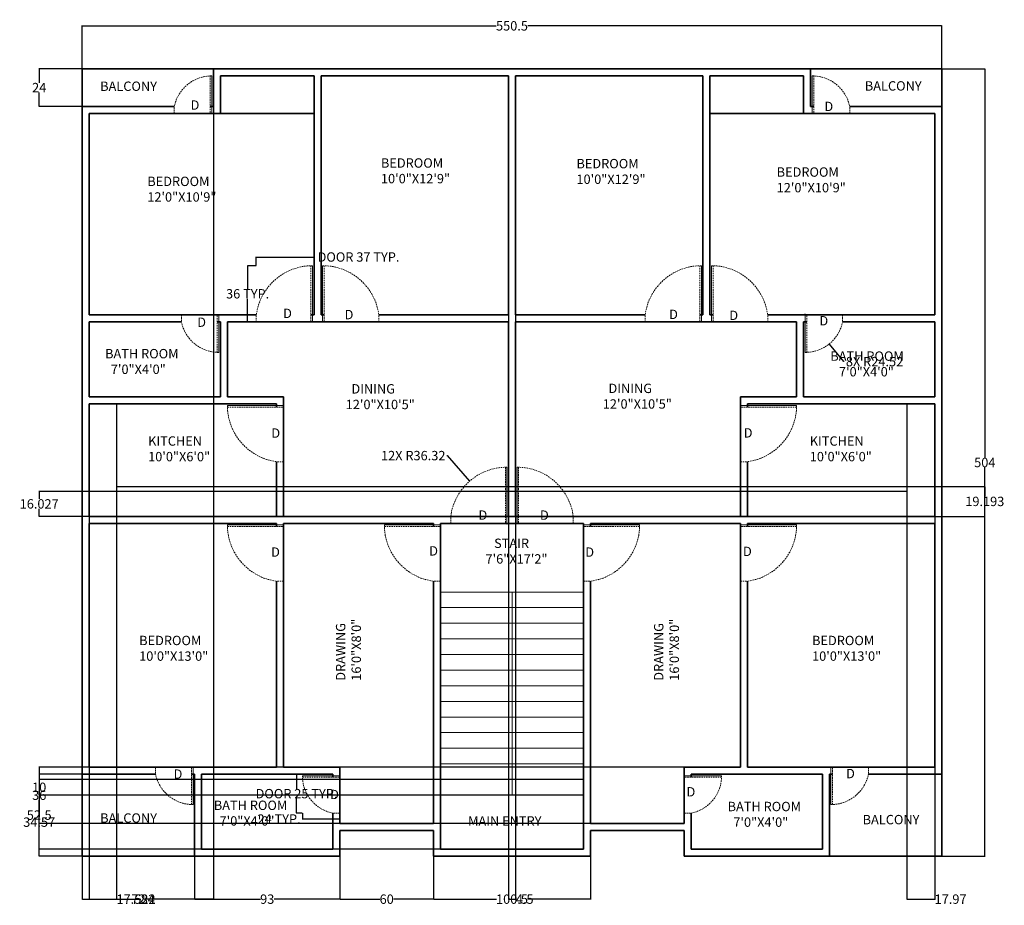
# Model space of a CAD drawing. Units: inches. Extents: x 4870 to 5501, y 14934 to 15501.
import ezdxf

# ---------------------------------------------------------------- set-up
doc = ezdxf.new("R2010")
doc.units = ezdxf.units.IN
doc.header["$MEASUREMENT"] = 0
doc.linetypes.add('DASHEDX2', pattern=[1.5, 1, -0.5])
for name, color, linetype, lineweight in [('A-ANNO-DIMS', 2, 'Continuous', 18), ('A-ANNO-TEXT', 7, 'Continuous', 18), ('A-AREA-IDEN', 7, 'Continuous', 18), ('A-DOOR', 4, 'DASHEDX2', 18), ('A-FLOR-FIXT', 8, 'Continuous', 18), ('A-FLOR-STRS', 7, 'Continuous', 18), ('A-WALL', 7, 'Continuous', 35)]:
    doc.layers.add(name, color=color, linetype=linetype, lineweight=lineweight)
doc.styles.get("Standard").update_dxf_attribs({"font": 'arial.ttf'})
doc.dimstyles.get("Standard").update_dxf_attribs({"dimtxt": 6, "dimasz": 0.18, "dimexe": 0.18, "dimexo": 0.0625, "dimgap": 0.09, "dimtad": 0, "dimtih": 1, "dimtoh": 1, "dimdec": 1, "dimzin": 0, "dimdsep": 46, "dimlunit": 3, "dimtxsty": 'Standard', "dimcen": 0.09, "dimadec": 0, "dimazin": 0, "dimtfac": 1, "dimtdec": 1, "dimtofl": 0, "dimtmove": 0, "dimatfit": 3, "dimfxl": 1, "dimtolj": 1, "dimtzin": 0, "dimarcsym": 0})

# ---------------------------------------------------------------- blocks, each defined once
blk = doc.blocks.new('DOOR-SWING-24IN')
for p, q in [((-1, 24), (-1, 0)), ((0, 0), (0, 24)), ((0, 24), (0, 0)), ((-24, 0), (-24, 4.5)), ((0, 0), (-24, 0)), ((1, 0), (0, 0))]:
    blk.add_line(p, q)
blk.add_arc((0, -0.52), 24.52, 90, 168.18772)
blk = doc.blocks.new('DOOR-SWING-36IN')
for p, q in [((-1, 36), (-1, 0)), ((0, 0), (0, 36)), ((0, 36), (0, 0)), ((-36, 0), (-36, 4.5)), ((0, 0), (-36, 0)), ((1, 0), (0, 0))]:
    blk.add_line(p, q)
blk.add_arc((0, -0.32), 36.32, 90, 172.37185)
blk = doc.blocks.new('*D3')
at = {"layer": 'A-ANNO-DIMS', "color": 0, "lineweight": -2, "transparency": 16777216}
for p, q in [((5021.91, 15343.26), (5021.91, 15348.93)), ((5022.09, 15348.75), (5058.73, 15348.75)), ((5058.91, 15343.26), (5058.91, 15348.93)), ((5058.91, 15348.75), (5059.09, 15348.75))]:
    blk.add_line(p, q, dxfattribs=at)
at = {"layer": 'A-ANNO-DIMS', "color": 0, "transparency": 16777216}
for points in [[(5022.09, 15348.78), (5022.09, 15348.72), (5021.91, 15348.75)], [(5058.73, 15348.78), (5058.73, 15348.72), (5058.91, 15348.75)]]:
    blk.add_solid(points, dxfattribs=at)
at = {"layer": 'Defpoints', "color": 0, "transparency": 16777216}
for p in [(5058.91, 15348.75), (5021.91, 15343.2), (5058.91, 15343.2)]:
    blk.add_point(p, dxfattribs=at)
at = {"layer": 'A-ANNO-DIMS', "color": 0, "transparency": 16777216, "insert": (5087.37, 15348.75), "char_height": 6, "attachment_point": 5}
blk.add_mtext('\\A1;DOOR 37 TYP.', dxfattribs=at)
blk = doc.blocks.new('*D4')
at = {"layer": 'A-ANNO-DIMS', "color": 0, "lineweight": -2, "transparency": 16777216}
for p, q in [((5021.85, 15343.2), (5016.18, 15343.2)), ((5016.36, 15343.02), (5016.36, 15328.35)), ((5016.36, 15307.38), (5016.36, 15322.04)), ((5021.85, 15307.2), (5016.18, 15307.2))]:
    blk.add_line(p, q, dxfattribs=at)
at = {"layer": 'A-ANNO-DIMS', "color": 0, "transparency": 16777216}
for points in [[(5016.33, 15343.02), (5016.39, 15343.02), (5016.36, 15343.2)], [(5016.33, 15307.38), (5016.39, 15307.38), (5016.36, 15307.2)]]:
    blk.add_solid(points, dxfattribs=at)
at = {"layer": 'Defpoints', "color": 0, "transparency": 16777216}
for p in [(5016.36, 15343.2), (5021.91, 15343.2), (5021.91, 15307.2)]:
    blk.add_point(p, dxfattribs=at)
at = {"layer": 'A-ANNO-DIMS', "color": 0, "transparency": 16777216, "insert": (5016.36, 15325.2), "char_height": 6, "attachment_point": 5}
blk.add_mtext('\\A1;36 TYP.', dxfattribs=at)
blk = doc.blocks.new('*D5')
at = {"layer": 'A-ANNO-DIMS', "color": 0, "lineweight": -2, "transparency": 16777216}
for p, q in [((5051.35, 15017.7), (5047.48, 15017.7)), ((5047.66, 15017.52), (5047.66, 15008.39)), ((5047.66, 14992.88), (5047.66, 15002)), ((5051.35, 14992.7), (5047.48, 14992.7))]:
    blk.add_line(p, q, dxfattribs=at)
at = {"layer": 'A-ANNO-DIMS', "color": 0, "transparency": 16777216}
for points in [[(5047.63, 15017.52), (5047.69, 15017.52), (5047.66, 15017.7)], [(5047.63, 14992.88), (5047.69, 14992.88), (5047.66, 14992.7)]]:
    blk.add_solid(points, dxfattribs=at)
at = {"layer": 'Defpoints', "color": 0, "transparency": 16777216}
for p in [(5047.66, 15017.7), (5051.41, 15017.7), (5051.41, 14992.7)]:
    blk.add_point(p, dxfattribs=at)
at = {"layer": 'A-ANNO-DIMS', "color": 0, "transparency": 16777216, "insert": (5047.66, 15005.2), "char_height": 6, "attachment_point": 5}
blk.add_mtext('\\A1;DOOR 25 TYP.', dxfattribs=at)
blk = doc.blocks.new('*D6')
at = {"layer": 'A-ANNO-DIMS', "color": 0, "lineweight": -2, "transparency": 16777216}
for p, q in [((5051.41, 14988.95), (5051.23, 14988.95)), ((5051.41, 14992.64), (5051.41, 14988.77)), ((5075.23, 14988.95), (5051.59, 14988.95)), ((5075.41, 14992.64), (5075.41, 14988.77))]:
    blk.add_line(p, q, dxfattribs=at)
at = {"layer": 'A-ANNO-DIMS', "color": 0, "transparency": 16777216}
for points in [[(5051.59, 14988.98), (5051.59, 14988.92), (5051.41, 14988.95)], [(5075.23, 14988.98), (5075.23, 14988.92), (5075.41, 14988.95)]]:
    blk.add_solid(points, dxfattribs=at)
at = {"layer": 'Defpoints', "color": 0, "transparency": 16777216}
for p in [(5051.41, 14992.7), (5051.41, 14988.95), (5075.41, 14992.7)]:
    blk.add_point(p, dxfattribs=at)
at = {"layer": 'A-ANNO-DIMS', "color": 0, "transparency": 16777216, "insert": (5036.49, 14988.95), "char_height": 6, "attachment_point": 5}
blk.add_mtext('\\A1;24 TYP.', dxfattribs=at)
blk = doc.blocks.new('*D7')
at = {"layer": 'A-ANNO-DIMS', "color": 0, "lineweight": -2, "transparency": 16777216}
for p, q in [((4910.41, 15469.26), (4910.41, 15496.91)), ((4910.59, 15496.73), (5175.43, 15496.73)), ((5460.73, 15496.73), (5195.9, 15496.73)), ((5460.91, 15469.26), (5460.91, 15496.91))]:
    blk.add_line(p, q, dxfattribs=at)
at = {"layer": 'A-ANNO-DIMS', "color": 0, "transparency": 16777216}
for points in [[(4910.59, 15496.76), (4910.59, 15496.7), (4910.41, 15496.73)], [(5460.73, 15496.76), (5460.73, 15496.7), (5460.91, 15496.73)]]:
    blk.add_solid(points, dxfattribs=at)
at = {"layer": 'Defpoints', "color": 0, "transparency": 16777216}
for p in [(5460.91, 15496.73), (4910.41, 15469.2), (5460.91, 15469.2)]:
    blk.add_point(p, dxfattribs=at)
at = {"layer": 'A-ANNO-DIMS', "color": 0, "transparency": 16777216, "insert": (5185.66, 15496.73), "char_height": 6, "attachment_point": 5}
blk.add_mtext('\\A1;550.5', dxfattribs=at)
blk = doc.blocks.new('*D8')
at = {"layer": 'A-ANNO-DIMS', "color": 0, "lineweight": -2, "transparency": 16777216}
for p, q in [((5460.97, 15469.2), (5488.62, 15469.2)), ((5488.44, 15469.02), (5488.44, 15220.35)), ((5488.44, 14965.38), (5488.44, 15214.04)), ((5460.97, 14965.2), (5488.62, 14965.2))]:
    blk.add_line(p, q, dxfattribs=at)
at = {"layer": 'A-ANNO-DIMS', "color": 0, "transparency": 16777216}
for points in [[(5488.41, 15469.02), (5488.47, 15469.02), (5488.44, 15469.2)], [(5488.41, 14965.38), (5488.47, 14965.38), (5488.44, 14965.2)]]:
    blk.add_solid(points, dxfattribs=at)
at = {"layer": 'Defpoints', "color": 0, "transparency": 16777216}
for p in [(5460.91, 15469.2), (5488.44, 15469.2), (5460.91, 14965.2)]:
    blk.add_point(p, dxfattribs=at)
at = {"layer": 'A-ANNO-DIMS', "color": 0, "transparency": 16777216, "insert": (5488.44, 15217.2), "char_height": 6, "attachment_point": 5}
blk.add_mtext('\\A1;504', dxfattribs=at)
blk = doc.blocks.new('*D9')
at = {"layer": 'A-ANNO-DIMS', "color": 0, "lineweight": -2, "transparency": 16777216}
for p, q in [((4910.41, 15469.14), (4910.41, 14937.49)), ((4994.41, 15469.14), (4994.41, 14937.49)), ((4910.59, 14937.67), (4948.03, 14937.67)), ((4994.23, 14937.67), (4956.79, 14937.67))]:
    blk.add_line(p, q, dxfattribs=at)
at = {"layer": 'A-ANNO-DIMS', "color": 0, "transparency": 16777216}
for points in [[(4910.59, 14937.7), (4910.59, 14937.64), (4910.41, 14937.67)], [(4994.23, 14937.7), (4994.23, 14937.64), (4994.41, 14937.67)]]:
    blk.add_solid(points, dxfattribs=at)
at = {"layer": 'Defpoints', "color": 0, "transparency": 16777216}
for p in [(4910.41, 15469.2), (4994.41, 15469.2), (4994.41, 14937.67)]:
    blk.add_point(p, dxfattribs=at)
at = {"layer": 'A-ANNO-DIMS', "color": 0, "transparency": 16777216, "insert": (4952.41, 14937.67), "char_height": 6, "attachment_point": 5}
blk.add_mtext('\\A1;84', dxfattribs=at)
blk = doc.blocks.new('*D10')
at = {"layer": 'A-ANNO-DIMS', "color": 0, "lineweight": -2, "transparency": 16777216}
for p, q in [((4910.35, 15469.2), (4882.7, 15469.2)), ((4882.88, 15469.02), (4882.88, 15460.3)), ((4882.88, 15445.38), (4882.88, 15454.1)), ((4910.35, 15445.2), (4882.7, 15445.2))]:
    blk.add_line(p, q, dxfattribs=at)
at = {"layer": 'A-ANNO-DIMS', "color": 0, "transparency": 16777216}
for points in [[(4882.85, 15469.02), (4882.91, 15469.02), (4882.88, 15469.2)], [(4882.85, 15445.38), (4882.91, 15445.38), (4882.88, 15445.2)]]:
    blk.add_solid(points, dxfattribs=at)
at = {"layer": 'Defpoints', "color": 0, "transparency": 16777216}
for p in [(4882.88, 15469.2), (4910.41, 15469.2), (4910.41, 15445.2)]:
    blk.add_point(p, dxfattribs=at)
at = {"layer": 'A-ANNO-DIMS', "color": 0, "transparency": 16777216, "insert": (4882.88, 15457.2), "char_height": 6, "attachment_point": 5}
blk.add_mtext('\\A1;24', dxfattribs=at)
blk = doc.blocks.new('*D11')
at = {"layer": 'A-ANNO-DIMS', "color": 0, "lineweight": -2, "transparency": 16777216}
for p, q in [((4910.41, 14965.14), (4910.41, 14937.49)), ((4982.41, 14965.14), (4982.41, 14937.49)), ((4910.59, 14937.67), (4942.08, 14937.67)), ((4982.23, 14937.67), (4950.74, 14937.67))]:
    blk.add_line(p, q, dxfattribs=at)
at = {"layer": 'A-ANNO-DIMS', "color": 0, "transparency": 16777216}
for points in [[(4910.59, 14937.7), (4910.59, 14937.64), (4910.41, 14937.67)], [(4982.23, 14937.7), (4982.23, 14937.64), (4982.41, 14937.67)]]:
    blk.add_solid(points, dxfattribs=at)
at = {"layer": 'Defpoints', "color": 0, "transparency": 16777216}
for p in [(4910.41, 14965.2), (4982.41, 14965.2), (4982.41, 14937.67)]:
    blk.add_point(p, dxfattribs=at)
at = {"layer": 'A-ANNO-DIMS', "color": 0, "transparency": 16777216, "insert": (4946.41, 14937.67), "char_height": 6, "attachment_point": 5}
blk.add_mtext('\\A1;72', dxfattribs=at)
blk = doc.blocks.new('*D12')
at = {"layer": 'A-ANNO-DIMS', "color": 0, "lineweight": -2, "transparency": 16777216}
for p, q in [((4910.35, 15017.7), (4882.7, 15017.7)), ((4882.88, 15017.52), (4882.88, 14994.6)), ((4882.88, 14965.38), (4882.88, 14988.29)), ((4910.35, 14965.2), (4882.7, 14965.2))]:
    blk.add_line(p, q, dxfattribs=at)
at = {"layer": 'A-ANNO-DIMS', "color": 0, "transparency": 16777216}
for points in [[(4882.85, 15017.52), (4882.91, 15017.52), (4882.88, 15017.7)], [(4882.85, 14965.38), (4882.91, 14965.38), (4882.88, 14965.2)]]:
    blk.add_solid(points, dxfattribs=at)
at = {"layer": 'Defpoints', "color": 0, "transparency": 16777216}
for p in [(4882.88, 15017.7), (4910.41, 15017.7), (4910.41, 14965.2)]:
    blk.add_point(p, dxfattribs=at)
at = {"layer": 'A-ANNO-DIMS', "color": 0, "transparency": 16777216, "insert": (4882.88, 14991.45), "char_height": 6, "attachment_point": 5}
blk.add_mtext('\\A1;52.5', dxfattribs=at)
blk = doc.blocks.new('*D13')
at = {"layer": 'A-ANNO-DIMS', "color": 0, "lineweight": -2, "transparency": 16777216}
for p, q in [((4982.41, 14965.14), (4982.41, 14937.49)), ((5075.41, 14965.14), (5075.41, 14937.49)), ((4982.59, 14937.67), (5024.52, 14937.67)), ((5075.23, 14937.67), (5033.3, 14937.67))]:
    blk.add_line(p, q, dxfattribs=at)
at = {"layer": 'A-ANNO-DIMS', "color": 0, "transparency": 16777216}
for points in [[(4982.59, 14937.7), (4982.59, 14937.64), (4982.41, 14937.67)], [(5075.23, 14937.7), (5075.23, 14937.64), (5075.41, 14937.67)]]:
    blk.add_solid(points, dxfattribs=at)
at = {"layer": 'Defpoints', "color": 0, "transparency": 16777216}
for p in [(4982.41, 14965.2), (5075.41, 14965.2), (5075.41, 14937.67)]:
    blk.add_point(p, dxfattribs=at)
at = {"layer": 'A-ANNO-DIMS', "color": 0, "transparency": 16777216, "insert": (5028.91, 14937.67), "char_height": 6, "attachment_point": 5}
blk.add_mtext('\\A1;93', dxfattribs=at)
blk = doc.blocks.new('*D14')
at = {"layer": 'A-ANNO-DIMS', "color": 0, "lineweight": -2, "transparency": 16777216}
for p, q in [((5075.41, 14965.14), (5075.41, 14937.49)), ((5135.41, 14965.14), (5135.41, 14937.49)), ((5075.59, 14937.67), (5101.02, 14937.67)), ((5135.23, 14937.67), (5109.81, 14937.67))]:
    blk.add_line(p, q, dxfattribs=at)
at = {"layer": 'A-ANNO-DIMS', "color": 0, "transparency": 16777216}
for points in [[(5075.59, 14937.7), (5075.59, 14937.64), (5075.41, 14937.67)], [(5135.23, 14937.7), (5135.23, 14937.64), (5135.41, 14937.67)]]:
    blk.add_solid(points, dxfattribs=at)
at = {"layer": 'Defpoints', "color": 0, "transparency": 16777216}
for p in [(5075.41, 14965.2), (5135.41, 14965.2), (5135.41, 14937.67)]:
    blk.add_point(p, dxfattribs=at)
at = {"layer": 'A-ANNO-DIMS', "color": 0, "transparency": 16777216, "insert": (5105.41, 14937.67), "char_height": 6, "attachment_point": 5}
blk.add_mtext('\\A1;60', dxfattribs=at)
blk = doc.blocks.new('*D15')
at = {"layer": 'A-ANNO-DIMS', "color": 0, "lineweight": -2, "transparency": 16777216}
for p, q in [((5135.41, 14965.14), (5135.41, 14937.49)), ((5235.91, 14965.14), (5235.91, 14937.49)), ((5135.59, 14937.67), (5175.71, 14937.67)), ((5235.73, 14937.67), (5195.62, 14937.67))]:
    blk.add_line(p, q, dxfattribs=at)
at = {"layer": 'A-ANNO-DIMS', "color": 0, "transparency": 16777216}
for points in [[(5135.59, 14937.7), (5135.59, 14937.64), (5135.41, 14937.67)], [(5235.73, 14937.7), (5235.73, 14937.64), (5235.91, 14937.67)]]:
    blk.add_solid(points, dxfattribs=at)
at = {"layer": 'Defpoints', "color": 0, "transparency": 16777216}
for p in [(5135.41, 14965.2), (5235.91, 14965.2), (5235.91, 14937.67)]:
    blk.add_point(p, dxfattribs=at)
at = {"layer": 'A-ANNO-DIMS', "color": 0, "transparency": 16777216, "insert": (5185.66, 14937.67), "char_height": 6, "attachment_point": 5}
blk.add_mtext('\\A1;100.5', dxfattribs=at)
blk = doc.blocks.new('*D16')
at = {"layer": 'A-ANNO-DIMS', "color": 0, "lineweight": -2, "transparency": 16777216}
for p, q in [((5295.85, 15022.2), (4882.7, 15022.2)), ((4882.88, 15022.02), (4882.88, 15007.35)), ((4882.88, 14986.38), (4882.88, 15001.04)), ((5295.85, 14986.2), (4882.7, 14986.2))]:
    blk.add_line(p, q, dxfattribs=at)
at = {"layer": 'A-ANNO-DIMS', "color": 0, "transparency": 16777216}
for points in [[(4882.85, 15022.02), (4882.91, 15022.02), (4882.88, 15022.2)], [(4882.85, 14986.38), (4882.91, 14986.38), (4882.88, 14986.2)]]:
    blk.add_solid(points, dxfattribs=at)
at = {"layer": 'Defpoints', "color": 0, "transparency": 16777216}
for p in [(4882.88, 15022.2), (5295.91, 15022.2), (5295.91, 14986.2)]:
    blk.add_point(p, dxfattribs=at)
at = {"layer": 'A-ANNO-DIMS', "color": 0, "transparency": 16777216, "insert": (4882.88, 15004.2), "char_height": 6, "attachment_point": 5}
blk.add_mtext('\\A1;36', dxfattribs=at)
blk = doc.blocks.new('*D17')
at = {"layer": 'A-ANNO-DIMS', "color": 0, "lineweight": -2, "transparency": 16777216}
for p, q in [((5231.35, 15004.27), (4882.7, 15004.27)), ((4882.88, 15004.09), (4882.88, 14990.14)), ((4882.88, 14969.88), (4882.88, 14983.83)), ((5231.35, 14969.7), (4882.7, 14969.7))]:
    blk.add_line(p, q, dxfattribs=at)
at = {"layer": 'A-ANNO-DIMS', "color": 0, "transparency": 16777216}
for points in [[(4882.85, 15004.09), (4882.91, 15004.09), (4882.88, 15004.27)], [(4882.85, 14969.88), (4882.91, 14969.88), (4882.88, 14969.7)]]:
    blk.add_solid(points, dxfattribs=at)
at = {"layer": 'Defpoints', "color": 0, "transparency": 16777216}
for p in [(4882.88, 15004.27), (5231.41, 15004.27), (5231.41, 14969.7)]:
    blk.add_point(p, dxfattribs=at)
at = {"layer": 'A-ANNO-DIMS', "color": 0, "transparency": 16777216, "insert": (4882.88, 14986.98), "char_height": 6, "attachment_point": 5}
blk.add_mtext('\\A1;34.57', dxfattribs=at)
blk = doc.blocks.new('*D18')
at = {"layer": 'A-ANNO-DIMS', "color": 0, "lineweight": -2, "transparency": 16777216}
for p, q in [((5231.35, 15014.27), (4882.7, 15014.27)), ((4882.88, 15014.09), (4882.88, 15012.42)), ((5231.35, 15004.27), (4882.7, 15004.27)), ((4882.88, 15004.45), (4882.88, 15006.12))]:
    blk.add_line(p, q, dxfattribs=at)
at = {"layer": 'A-ANNO-DIMS', "color": 0, "transparency": 16777216}
for points in [[(4882.85, 15014.09), (4882.91, 15014.09), (4882.88, 15014.27)], [(4882.85, 15004.45), (4882.91, 15004.45), (4882.88, 15004.27)]]:
    blk.add_solid(points, dxfattribs=at)
at = {"layer": 'Defpoints', "color": 0, "transparency": 16777216}
for p in [(4882.88, 15014.27), (5231.41, 15014.27), (5231.41, 15004.27)]:
    blk.add_point(p, dxfattribs=at)
at = {"layer": 'A-ANNO-DIMS', "color": 0, "transparency": 16777216, "insert": (4882.88, 15009.27), "char_height": 6, "attachment_point": 5}
blk.add_mtext('\\A1;10', dxfattribs=at)
blk = doc.blocks.new('*D19')
at = {"layer": 'A-ANNO-DIMS', "color": 0, "lineweight": -2, "transparency": 16777216}
for p, q in [((5183.41, 15464.64), (5183.41, 14937.49)), ((5187.91, 15464.64), (5187.91, 14937.49)), ((5183.59, 14937.67), (5187.73, 14937.67)), ((5187.91, 14937.67), (5188.09, 14937.67))]:
    blk.add_line(p, q, dxfattribs=at)
at = {"layer": 'A-ANNO-DIMS', "color": 0, "transparency": 16777216}
for points in [[(5183.59, 14937.7), (5183.59, 14937.64), (5183.41, 14937.67)], [(5187.73, 14937.7), (5187.73, 14937.64), (5187.91, 14937.67)]]:
    blk.add_solid(points, dxfattribs=at)
at = {"layer": 'Defpoints', "color": 0, "transparency": 16777216}
for p in [(5183.41, 15464.7), (5187.91, 15464.7), (5187.91, 14937.67)]:
    blk.add_point(p, dxfattribs=at)
at = {"layer": 'A-ANNO-DIMS', "color": 0, "transparency": 16777216, "insert": (5193.79, 14937.67), "char_height": 6, "attachment_point": 5}
blk.add_mtext('\\A1;4.5', dxfattribs=at)
blk = doc.blocks.new('*D20')
at = {"layer": 'A-ANNO-DIMS', "color": 0, "lineweight": -2, "transparency": 16777216}
for p, q in [((4914.91, 15254.64), (4914.91, 14937.49)), ((4932.43, 15254.64), (4932.43, 14937.49)), ((4915.09, 14937.67), (4932.25, 14937.67)), ((4932.43, 14937.67), (4932.61, 14937.67))]:
    blk.add_line(p, q, dxfattribs=at)
at = {"layer": 'A-ANNO-DIMS', "color": 0, "transparency": 16777216}
for points in [[(4915.09, 14937.7), (4915.09, 14937.64), (4914.91, 14937.67)], [(4932.25, 14937.7), (4932.25, 14937.64), (4932.43, 14937.67)]]:
    blk.add_solid(points, dxfattribs=at)
at = {"layer": 'Defpoints', "color": 0, "transparency": 16777216}
for p in [(4914.91, 15254.7), (4932.43, 15254.7), (4932.43, 14937.67)]:
    blk.add_point(p, dxfattribs=at)
at = {"layer": 'A-ANNO-DIMS', "color": 0, "transparency": 16777216, "insert": (4944.85, 14937.67), "char_height": 6, "attachment_point": 5}
blk.add_mtext('\\A1;17.522', dxfattribs=at)
blk = doc.blocks.new('*D21')
at = {"layer": 'A-ANNO-DIMS', "color": 0, "lineweight": -2, "transparency": 16777216}
for p, q in [((4932.5, 15201.89), (5488.62, 15201.89)), ((5488.44, 15201.71), (5488.44, 15195.45)), ((5488.44, 15182.88), (5488.44, 15189.14)), ((4914.97, 15182.7), (5488.62, 15182.7))]:
    blk.add_line(p, q, dxfattribs=at)
at = {"layer": 'A-ANNO-DIMS', "color": 0, "transparency": 16777216}
for points in [[(5488.41, 15201.71), (5488.47, 15201.71), (5488.44, 15201.89)], [(5488.41, 15182.88), (5488.47, 15182.88), (5488.44, 15182.7)]]:
    blk.add_solid(points, dxfattribs=at)
at = {"layer": 'Defpoints', "color": 0, "transparency": 16777216}
for p in [(4932.43, 15201.89), (5488.44, 15201.89), (4914.91, 15182.7)]:
    blk.add_point(p, dxfattribs=at)
at = {"layer": 'A-ANNO-DIMS', "color": 0, "transparency": 16777216, "insert": (5488.44, 15192.29), "char_height": 6, "attachment_point": 5}
blk.add_mtext('\\A1;19.193', dxfattribs=at)
blk = doc.blocks.new('*D22')
at = {"layer": 'A-ANNO-DIMS', "color": 0, "lineweight": -2, "transparency": 16777216}
for p, q in [((5438.44, 15254.64), (5438.44, 14937.49)), ((5456.41, 15254.64), (5456.41, 14937.49)), ((5438.62, 14937.67), (5456.23, 14937.67)), ((5456.41, 14937.67), (5456.59, 14937.67))]:
    blk.add_line(p, q, dxfattribs=at)
at = {"layer": 'A-ANNO-DIMS', "color": 0, "transparency": 16777216}
for points in [[(5438.62, 14937.7), (5438.62, 14937.64), (5438.44, 14937.67)], [(5456.23, 14937.7), (5456.23, 14937.64), (5456.41, 14937.67)]]:
    blk.add_solid(points, dxfattribs=at)
at = {"layer": 'Defpoints', "color": 0, "transparency": 16777216}
for p in [(5438.44, 15254.7), (5456.41, 15254.7), (5456.41, 14937.67)]:
    blk.add_point(p, dxfattribs=at)
at = {"layer": 'A-ANNO-DIMS', "color": 0, "transparency": 16777216, "insert": (5466.52, 14937.67), "char_height": 6, "attachment_point": 5}
blk.add_mtext('\\A1;17.97', dxfattribs=at)
blk = doc.blocks.new('*D23')
at = {"layer": 'A-ANNO-DIMS', "color": 0, "lineweight": -2, "transparency": 16777216}
for p, q in [((5438.38, 15198.73), (4882.7, 15198.73)), ((4882.88, 15198.55), (4882.88, 15193.86)), ((4882.88, 15182.88), (4882.88, 15187.56)), ((5456.35, 15182.7), (4882.7, 15182.7))]:
    blk.add_line(p, q, dxfattribs=at)
at = {"layer": 'A-ANNO-DIMS', "color": 0, "transparency": 16777216}
for points in [[(4882.85, 15198.55), (4882.91, 15198.55), (4882.88, 15198.73)], [(4882.85, 15182.88), (4882.91, 15182.88), (4882.88, 15182.7)]]:
    blk.add_solid(points, dxfattribs=at)
at = {"layer": 'Defpoints', "color": 0, "transparency": 16777216}
for p in [(5438.44, 15198.73), (4882.88, 15182.7), (5456.41, 15182.7)]:
    blk.add_point(p, dxfattribs=at)
at = {"layer": 'A-ANNO-DIMS', "color": 0, "transparency": 16777216, "insert": (4882.88, 15190.71), "char_height": 6, "attachment_point": 5}
blk.add_mtext('\\A1;16.027', dxfattribs=at)
blk = doc.blocks.new('*D24')
at = {"layer": 'A-ANNO-DIMS', "color": 0, "lineweight": -2, "transparency": 16777216}
for p, q in [((5143.96, 15221.61), (5144.14, 15221.61)), ((5144.14, 15221.61), (5158.38, 15205.35)), ((5182.32, 15177.88), (5182.5, 15177.88)), ((5182.41, 15177.79), (5182.41, 15177.97))]:
    blk.add_line(p, q, dxfattribs=at)
at = {"layer": 'A-ANNO-DIMS', "color": 0, "transparency": 16777216}
blk.add_solid([(5158.4, 15205.37), (5158.35, 15205.33), (5158.49, 15205.21)], dxfattribs=at)
at = {"layer": 'Defpoints', "color": 0, "transparency": 16777216}
for p in [(5158.49, 15205.21), (5182.41, 15177.88)]:
    blk.add_point(p, dxfattribs=at)
at = {"layer": 'A-ANNO-DIMS', "color": 0, "transparency": 16777216, "insert": (5122.41, 15221.61), "char_height": 6, "attachment_point": 5}
blk.add_mtext('\\A1;12X R36.32', dxfattribs=at)
blk = doc.blocks.new('*D25')
at = {"layer": 'A-ANNO-DIMS', "color": 0, "lineweight": -2, "transparency": 16777216}
for p, q in [((5373.32, 15312.22), (5373.5, 15312.22)), ((5373.41, 15312.13), (5373.41, 15312.31)), ((5398.15, 15281.77), (5388.99, 15293.05)), ((5398.33, 15281.77), (5398.15, 15281.77))]:
    blk.add_line(p, q, dxfattribs=at)
at = {"layer": 'A-ANNO-DIMS', "color": 0, "transparency": 16777216}
blk.add_solid([(5389.01, 15293.07), (5388.96, 15293.03), (5388.87, 15293.19)], dxfattribs=at)
at = {"layer": 'Defpoints', "color": 0, "transparency": 16777216}
for p in [(5373.41, 15312.22), (5388.87, 15293.19)]:
    blk.add_point(p, dxfattribs=at)
at = {"layer": 'A-ANNO-DIMS', "color": 0, "transparency": 16777216, "insert": (5417.83, 15281.77), "char_height": 6, "attachment_point": 5}
blk.add_mtext('\\A1;8X R24.52', dxfattribs=at)

msp = doc.modelspace()

# ---------------------------------------------------------------- linework, layer by layer
at = {"layer": 'A-FLOR-FIXT'}
for p, q in [((4932.4343, 15254.6978), (4932.4343, 15201.891)), ((5438.4417, 15254.6978), (5438.4417, 15198.7253)), ((4932.4343, 15201.891), (5034.9123, 15201.891)), ((5438.4417, 15198.7253), (5336.4123, 15198.7253))]:
    msp.add_line(p, q, dxfattribs=at)
at = {"layer": 'A-FLOR-STRS'}
for p, q in [((5139.9123, 15134.2693), (5231.4123, 15134.2693)), ((5185.6623, 15134.2693), (5185.6623, 15004.2693)), ((5139.9123, 15124.2693), (5231.4123, 15124.2693)), ((5139.9123, 15114.2693), (5231.4123, 15114.2693)), ((5139.9123, 15104.2693), (5231.4123, 15104.2693)), ((5139.9123, 15094.2693), (5231.4123, 15094.2693)), ((5139.9123, 15084.2693), (5231.4123, 15084.2693)), ((5139.9123, 15074.2693), (5231.4123, 15074.2693)), ((5139.9123, 15064.2693), (5231.4123, 15064.2693)), ((5139.9123, 15054.2693), (5231.4123, 15054.2693)), ((5139.9123, 15044.2693), (5231.4123, 15044.2693)), ((5139.9123, 15034.2693), (5231.4123, 15034.2693)), ((5139.9123, 15024.2693), (5231.4123, 15024.2693)), ((5139.9123, 15014.2693), (5231.4123, 15014.2693)), ((5139.9123, 15004.2693), (5231.4123, 15004.2693))]:
    msp.add_line(p, q, dxfattribs=at)
at = {"layer": 'A-WALL'}
for p, q in [((4910.4123, 15469.1978), (5460.9123, 15469.1978)), ((4910.4123, 15469.1978), (4910.4123, 14965.1978)), ((4994.4123, 15469.1978), (4994.4123, 15445.1978)), ((5376.9123, 15469.1978), (5376.9123, 15445.1978)), ((5460.9123, 15469.1978), (5460.9123, 14965.1978)), ((4998.9123, 15464.6978), (5058.9123, 15464.6978)), ((4998.9123, 15464.6978), (4998.9123, 15440.6978)), ((4998.9123, 15464.6978), (5058.9123, 15464.6978)), ((5058.9123, 15464.6978), (5058.9123, 15311.6978)), ((5063.4123, 15464.6978), (5063.4123, 15311.6978)), ((5063.4123, 15464.6978), (5183.4123, 15464.6978)), ((5183.4123, 15464.6978), (5183.4123, 15311.6978)), ((5187.9123, 15464.6978), (5187.9123, 15311.6978)), ((5187.9123, 15464.6978), (5307.9123, 15464.6978)), ((5307.9123, 15464.6978), (5307.9123, 15311.6978)), ((5312.4123, 15464.6978), (5312.4123, 15311.6978)), ((5312.4123, 15464.6978), (5372.4123, 15464.6978)), ((5372.4123, 15464.6978), (5372.4123, 15440.6978)), ((4910.4123, 15445.1978), (4969.4123, 15445.1978)), ((4992.4123, 15445.1978), (4994.4123, 15445.1978)), ((5376.9123, 15445.1978), (5378.9123, 15445.1978)), ((5401.9123, 15445.1978), (5460.9123, 15445.1978)), ((4914.9123, 15440.6978), (5058.9123, 15440.6978)), ((4914.9123, 15440.6978), (4914.9123, 15311.6978)), ((5312.4123, 15440.6978), (5456.4123, 15440.6978)), ((5456.4123, 15440.6978), (5456.4123, 15311.6978)), ((4914.9123, 15311.6978), (5021.9123, 15311.6978)), ((5056.9123, 15311.6978), (5058.9123, 15311.6978)), ((5063.4123, 15311.6978), (5065.4123, 15311.6978)), ((5100.4123, 15311.6978), (5183.4123, 15311.6978)), ((5187.9123, 15311.6978), (5270.9123, 15311.6978)), ((5305.9123, 15311.6978), (5307.9123, 15311.6978)), ((5312.4123, 15311.6978), (5314.4123, 15311.6978)), ((5349.4123, 15311.6978), (5456.4123, 15311.6978)), ((4914.9123, 15307.1978), (4973.9123, 15307.1978)), ((4914.9123, 15307.1978), (4914.9123, 15259.1978)), ((4996.9123, 15307.1978), (4998.9123, 15307.1978)), ((4998.9123, 15307.1978), (4998.9123, 15259.1978)), ((5003.4123, 15307.1978), (5003.4123, 15259.1978)), ((5003.4123, 15307.1978), (5183.4123, 15307.1978)), ((5183.4123, 15307.1978), (5183.4123, 15182.6978)), ((5187.9123, 15307.1978), (5187.9123, 15182.6978)), ((5187.9123, 15307.1978), (5367.9123, 15307.1978)), ((5367.9123, 15307.1978), (5367.9123, 15259.1978)), ((5372.4123, 15307.1978), (5372.4123, 15259.1978)), ((5372.4123, 15307.1978), (5374.4123, 15307.1978)), ((5397.4123, 15307.1978), (5456.4123, 15307.1978)), ((5456.4123, 15307.1978), (5456.4123, 15259.1978)), ((4914.9123, 15259.1978), (4998.9123, 15259.1978)), ((4914.9123, 15259.1978), (4998.9123, 15259.1978)), ((4914.9123, 15254.6978), (5034.9123, 15254.6978)), ((4914.9123, 15254.6978), (5034.9123, 15254.6978)), ((4914.9123, 15254.6978), (4914.9123, 15182.6978)), ((5003.4123, 15259.1978), (5039.4123, 15259.1978)), ((5003.4123, 15259.1978), (5039.4123, 15259.1978)), ((5034.9123, 15254.6978), (5034.9123, 15252.6978)), ((5039.4123, 15259.1978), (5039.4123, 15182.6978)), ((5331.9123, 15259.1978), (5367.9123, 15259.1978)), ((5331.9123, 15259.1978), (5331.9123, 15182.6978)), ((5336.4123, 15254.6978), (5456.4123, 15254.6978)), ((5336.4123, 15254.6978), (5336.4123, 15252.6978)), ((5372.4123, 15259.1978), (5456.4123, 15259.1978)), ((5456.4123, 15254.6978), (5456.4123, 15182.6978)), ((5034.9123, 15217.6978), (5034.9123, 15182.6978)), ((5336.4123, 15217.6978), (5336.4123, 15182.6978)), ((4914.9123, 15182.6978), (5034.9123, 15182.6978)), ((4914.9123, 15178.1978), (5034.9123, 15178.1978)), ((4914.9123, 15178.1978), (4914.9123, 15022.1978)), ((5034.9123, 15178.1978), (5034.9123, 15176.1978)), ((5039.4123, 15182.6978), (5146.4123, 15182.6978)), ((5039.4123, 15178.1978), (5039.4123, 15022.1978)), ((5039.4123, 15178.1978), (5135.4123, 15178.1978)), ((5135.4123, 15178.1978), (5135.4123, 15176.1978)), ((5139.9123, 15178.1978), (5139.9123, 14969.6978)), ((5139.9123, 15178.1978), (5231.4123, 15178.1978)), ((5181.4123, 15182.6978), (5183.4123, 15182.6978)), ((5187.9123, 15182.6978), (5189.9123, 15182.6978)), ((5224.9123, 15182.6978), (5331.9123, 15182.6978)), ((5231.4123, 15178.1978), (5231.4123, 14969.6978)), ((5235.9123, 15178.1978), (5235.9123, 15176.1978)), ((5235.9123, 15178.1978), (5331.9123, 15178.1978)), ((5331.9123, 15178.1978), (5331.9123, 15022.1978)), ((5336.4123, 15182.6978), (5456.4123, 15182.6978)), ((5336.4123, 15178.1978), (5456.4123, 15178.1978)), ((5336.4123, 15178.1978), (5336.4123, 15176.1978)), ((5456.4123, 15178.1978), (5456.4123, 15022.1978)), ((5034.9123, 15141.1978), (5034.9123, 15022.1978)), ((5135.4123, 15141.1978), (5135.4123, 14986.1978)), ((5235.9123, 15141.1978), (5235.9123, 14986.1978)), ((5336.4123, 15141.1978), (5336.4123, 15022.1978)), ((4914.9123, 15022.1978), (5034.9123, 15022.1978)), ((5039.4123, 15022.1978), (5075.4123, 15022.1978)), ((5075.4123, 15022.1978), (5075.4123, 14986.1978)), ((5295.9123, 15022.1978), (5331.9123, 15022.1978)), ((5295.9123, 15022.1978), (5295.9123, 14986.1978)), ((5336.4123, 15022.1978), (5456.4123, 15022.1978)), ((4914.9123, 15017.6978), (4910.4123, 15017.6978)), ((4914.9123, 15017.6978), (4957.4123, 15017.6978)), ((4980.4123, 15017.6978), (4982.4123, 15017.6978)), ((4982.4123, 15017.6978), (4982.4123, 14969.6978)), ((4986.9123, 15017.6978), (4986.9123, 14969.6978)), ((4986.9123, 15017.6978), (5070.9123, 15017.6978)), ((5070.9123, 15017.6978), (5070.9123, 15015.6978)), ((5300.4123, 15017.6978), (5384.4123, 15017.6978)), ((5300.4123, 15017.6978), (5300.4123, 15015.6978)), ((5384.4123, 15017.6978), (5384.4123, 14969.6978)), ((5388.9123, 15017.6978), (5388.9123, 14969.6978)), ((5388.9123, 15017.6978), (5390.9123, 15017.6978)), ((5413.9123, 15017.6978), (5456.4123, 15017.6978)), ((5456.4123, 15017.6978), (5460.9123, 15017.6978)), ((5070.9123, 14992.6978), (5070.9123, 14969.6978)), ((5300.4123, 14992.6978), (5300.4123, 14969.6978)), ((5075.4123, 14986.1978), (5135.4123, 14986.1978)), ((5235.9123, 14986.1978), (5295.9123, 14986.1978)), ((5075.4123, 14981.6978), (5135.4123, 14981.6978)), ((5075.4123, 14981.6978), (5075.4123, 14965.1978)), ((5135.4123, 14981.6978), (5135.4123, 14965.1978)), ((5235.9123, 14981.6978), (5295.9123, 14981.6978)), ((5235.9123, 14981.6978), (5235.9123, 14965.1978)), ((5295.9123, 14981.6978), (5295.9123, 14965.1978)), ((4982.4123, 14969.6978), (4982.4123, 14965.1978)), ((4986.9123, 14969.6978), (5070.9123, 14969.6978)), ((5139.9123, 14969.6978), (5231.4123, 14969.6978)), ((5300.4123, 14969.6978), (5384.4123, 14969.6978)), ((5388.9123, 14969.6978), (5388.9123, 14965.1978)), ((4910.4123, 14965.1978), (5075.4123, 14965.1978)), ((5135.4123, 14965.1978), (5235.9123, 14965.1978)), ((5295.9123, 14965.1978), (5460.9123, 14965.1978))]:
    msp.add_line(p, q, dxfattribs=at)

# ---------------------------------------------------------------- block references
at = {"layer": 'A-DOOR'}
for name, p in [('DOOR-SWING-24IN', (4993.4123, 15440.6978)), ('DOOR-SWING-36IN', (5057.9123, 15307.1978)), ('DOOR-SWING-36IN', (5306.9123, 15307.1978)), ('DOOR-SWING-36IN', (5182.4123, 15178.1978))]:
    msp.add_blockref(name, p, dxfattribs=at)
at = {"layer": 'A-DOOR', "extrusion": (0, 0, -1), "zscale": -1}
for name, p in [('DOOR-SWING-24IN', (-5377.9123, 15440.6978)), ('DOOR-SWING-36IN', (-5064.4123, 15307.1978)), ('DOOR-SWING-36IN', (-5313.4123, 15307.1978)), ('DOOR-SWING-36IN', (-5188.9123, 15178.1978))]:
    msp.add_blockref(name, p, dxfattribs=at)
for name, p, rotation in [('DOOR-SWING-24IN', (-4997.9123, 15311.6978), 180), ('DOOR-SWING-36IN', (-5331.9123, 15253.6978), 89.99999999999628), ('DOOR-SWING-36IN', (-5231.4123, 15177.1978), 89.99999999999454), ('DOOR-SWING-36IN', (-5331.9123, 15177.1978), 89.99999999999628), ('DOOR-SWING-24IN', (-4981.4123, 15022.1978), 180), ('DOOR-SWING-24IN', (-5295.9123, 15016.6978), 89.99999999999078)]:
    msp.add_blockref(name, p, dxfattribs=dict(at, rotation=rotation))
at = {"layer": 'A-DOOR'}
for name, p, rotation in [('DOOR-SWING-24IN', (5373.4123, 15311.6978), 180), ('DOOR-SWING-36IN', (5039.4123, 15253.6978), 89.999999999998), ('DOOR-SWING-36IN', (5039.4123, 15177.1978), 89.99999999999628), ('DOOR-SWING-36IN', (5139.9123, 15177.1978), 89.99999999999459), ('DOOR-SWING-24IN', (5389.9123, 15022.1978), 180), ('DOOR-SWING-24IN', (5075.4123, 15016.6978), 89.99999999998566)]:
    msp.add_blockref(name, p, dxfattribs=dict(at, rotation=rotation))

# ---------------------------------------------------------------- texts
at = {"layer": 'A-ANNO-TEXT', "char_height": 6, "attachment_point": 1}
for insert in [(4979.8128, 15449.0312), (5385.7132, 15448.1439), (4984.077, 15310.0205), (5039.0588, 15315.677), (5078.4574, 15314.8863), (5286.2544, 15315.0432), (5324.8466, 15314.4074), (5382.5175, 15310.946), (5031.5547, 15239.0229), (5334.0601, 15239.1591), (5164.1882, 15186.5349), (5203.5882, 15186.504), (5031.3647, 15162.8669), (5132.6289, 15163.6286), (5232.5929, 15162.828), (5333.6042, 15163.298), (4968.925, 15020.7318), (5399.5923, 15021.068), (5069.1859, 15007.6837), (5297.412, 15009.3914)]:
    msp.add_mtext_dynamic_manual_height_columns('D', width=9.293401, gutter_width=30, heights=[0], dxfattribs=dict(at, insert=insert))
at = {"layer": 'A-AREA-IDEN', "char_height": 6, "attachment_point": 1}
for s, width, insert in [('BALCONY', 43.463843, (4921.9382, 15461.0657)), ('BALCONY', 42.36689, (5411.6287, 15461.2764)), ('BEDROOM\\P10\'0"X12\'9"', 54.993986, (5101.735, 15411.9288)), ('BEDROOM\\P10\'0"X12\'9"', 75.741013, (5226.9316, 15411.5267)), ('BEDROOM\\P12\'0"X10\'9"', 64.22061, (5355.1472, 15406.1399)), ('BEDROOM\\P12\'0"X10\'9"', 76.737164, (4952.1044, 15400.1757)), ('BATH ROOM\\P  7\'0"X4\'0"', 51.687203, (4925.079, 15289.8765)), ('BATH ROOM\\P   7\'0"X4\'0"', 62.004808, (5389.5282, 15288.3083)), ('  DINING\\P12\'0"X10\'5"', 68.873434, (5079.1633, 15267.3462)), ('  DINING\\P12\'0"X10\'5"', 68.873434, (5243.785, 15267.6653)), ('KITCHEN\\P10\'0"X6\'0"', 60.117128, (4952.6317, 15233.9598)), ('KITCHEN\\P10\'0"X6\'0"', 60.117128, (5376.3513, 15233.9598)), ('   STAIR\\P7\'6"X17\'2"', 39.53126, (5168.698, 15168.4795)), ('BEDROOM\\P10\'0"X13\'0"', 63.399481, (4946.8944, 15106.2661)), ('BEDROOM\\P10\'0"X13\'0"', 63.399481, (5377.8204, 15106.2661)), ('BATH ROOM\\P  7\'0"X4\'0"', 51.687203, (4994.7112, 15000.744)), ('BATH ROOM\\P  7\'0"X4\'0"', 51.687203, (5323.7384, 14999.9754)), ('BALCONY', 43.463843, (4921.9382, 14992.5967)), ('MAIN ENTRY', 79.450475, (5157.5552, 14990.7304)), ('BALCONY', 43.463843, (5410.2171, 14991.5837))]:
    msp.add_mtext_dynamic_manual_height_columns(s, width=width, gutter_width=30, heights=[0], dxfattribs=dict(at, insert=insert))
at = {"layer": 'A-AREA-IDEN', "char_height": 6, "attachment_point": 1, "rotation": 90}
for insert in [(5072.9248, 15077.476), (5276.6133, 15077.476)]:
    msp.add_mtext_dynamic_manual_height_columns('DRAWING\\P16\'0"X8\'0"', width=50.452667, gutter_width=30, heights=[0], dxfattribs=dict(at, insert=insert))

# ---------------------------------------------------------------- dimensions: what is measured, and where the dimension line sits
at = {"layer": 'A-ANNO-DIMS'}
for base, p1, p2, override, picture, middle in [((5460.9123, 15496.7253), (4910.4123, 15469.1978), (5460.9123, 15469.1978), {"dimdec": 1, "dimlfac": 1, "dimrnd": 0, "dimzin": 0, "dimdsep": 46, "dimlunit": 2}, '*D7', (5185.6623, 15496.7253)), ((4994.4123, 14937.6703), (4910.4123, 15469.1978), (4994.4123, 15469.1978), {"dimdec": 0, "dimlfac": 1, "dimrnd": 0, "dimzin": 0, "dimdsep": 46, "dimlunit": 2}, '*D9', (4952.4123, 14937.6703)), ((5187.9123, 14937.6703), (5183.4123, 15464.6978), (5187.9123, 15464.6978), {"dimdec": 1, "dimlfac": 1, "dimrnd": 0, "dimzin": 0, "dimdsep": 46, "dimlunit": 2}, '*D19', (5193.7873, 14937.6703)), ((4932.4343, 14937.6703), (4914.9123, 15254.6978), (4932.4343, 15254.6978), {"dimdec": 3, "dimlfac": 1, "dimrnd": 0, "dimzin": 0, "dimdsep": 46, "dimlunit": 2}, '*D20', (4944.8455, 14937.6703)), ((5456.4123, 14937.6703), (5438.4417, 15254.6978), (5456.4123, 15254.6978), {"dimdec": 2, "dimlfac": 1, "dimrnd": 0, "dimzin": 0, "dimdsep": 46, "dimlunit": 2}, '*D22', (5466.5233, 14937.6703)), ((4982.4123, 14937.6703), (4910.4123, 14965.1978), (4982.4123, 14965.1978), {"dimdec": 0, "dimlfac": 1, "dimrnd": 0, "dimzin": 0, "dimdsep": 46, "dimlunit": 2}, '*D11', (4946.4123, 14937.6703)), ((5075.4123, 14937.6703), (4982.4123, 14965.1978), (5075.4123, 14965.1978), {"dimdec": 0, "dimlfac": 1, "dimrnd": 0, "dimzin": 0, "dimdsep": 46, "dimlunit": 2}, '*D13', (5028.9123, 14937.6703)), ((5135.4123, 14937.6703), (5075.4123, 14965.1978), (5135.4123, 14965.1978), {"dimdec": 0, "dimlfac": 1, "dimrnd": 0, "dimzin": 0, "dimdsep": 46, "dimlunit": 2}, '*D14', (5105.4123, 14937.6703)), ((5235.9123, 14937.6703), (5135.4123, 14965.1978), (5235.9123, 14965.1978), {"dimdec": 1, "dimlfac": 1, "dimrnd": 0, "dimzin": 0, "dimdsep": 46, "dimlunit": 2}, '*D15', (5185.6623, 14937.6703))]:
    dim = msp.add_linear_dim(base=base, p1=p1, p2=p2, dimstyle='Standard', override=override, dxfattribs=at)
    dim.commit()
    dim.dimension.update_dxf_attribs({"geometry": picture, "text_midpoint": middle})
for base, p1, p2, override, picture, middle in [((4882.8848, 15469.1978), (4910.4123, 15445.1978), (4910.4123, 15469.1978), {"dimdec": 0, "dimlfac": 1, "dimrnd": 0, "dimzin": 0, "dimdsep": 46, "dimlunit": 2}, '*D10', (4882.8848, 15457.1978)), ((5488.4398, 15469.1978), (5460.9123, 14965.1978), (5460.9123, 15469.1978), {"dimdec": 0, "dimlfac": 1, "dimrnd": 0, "dimzin": 0, "dimdsep": 46, "dimlunit": 2}, '*D8', (5488.4398, 15217.1978)), ((4882.88475, 15182.69779), (5438.44166, 15198.72525), (5456.41225, 15182.69779), {"dimdec": 3, "dimlfac": 1, "dimrnd": 0, "dimzin": 0, "dimdsep": 46, "dimlunit": 2}, '*D23', (4882.88475, 15190.71152)), ((5488.4398, 15201.891), (4914.9123, 15182.6978), (4932.4343, 15201.891), {"dimdec": 3, "dimlfac": 1, "dimrnd": 0, "dimzin": 0, "dimdsep": 46, "dimlunit": 2}, '*D21', (5488.4398, 15192.2944)), ((4882.8848, 15022.1978), (5295.9123, 14986.1978), (5295.9123, 15022.1978), {"dimdec": 0, "dimlfac": 1, "dimrnd": 0, "dimzin": 0, "dimdsep": 46, "dimlunit": 2}, '*D16', (4882.8848, 15004.1978)), ((4882.8848, 15017.6978), (4910.4123, 14965.1978), (4910.4123, 15017.6978), {"dimdec": 1, "dimlfac": 1, "dimrnd": 0, "dimzin": 0, "dimdsep": 46, "dimlunit": 2}, '*D12', (4882.8848, 14991.4478)), ((4882.8848, 15014.2693), (5231.4123, 15004.2693), (5231.4123, 15014.2693), {"dimdec": 0, "dimlfac": 1, "dimrnd": 0, "dimzin": 0, "dimdsep": 46, "dimlunit": 2}, '*D18', (4882.8848, 15009.2693)), ((4882.8848, 15004.2693), (5231.4123, 14969.6978), (5231.4123, 15004.2693), {"dimdec": 2, "dimlfac": 1, "dimrnd": 0, "dimzin": 0, "dimdsep": 46, "dimlunit": 2}, '*D17', (4882.8848, 14986.9835))]:
    dim = msp.add_linear_dim(base=base, p1=p1, p2=p2, angle=90, dimstyle='Standard', override=override, dxfattribs=at)
    dim.commit()
    dim.dimension.update_dxf_attribs({"geometry": picture, "text_midpoint": middle})
dim = msp.add_linear_dim(base=(5058.9123, 15348.7478), p1=(5021.9123, 15343.1978), p2=(5058.9123, 15343.1978), text='DOOR <> TYP.', dimstyle='Standard', override={"dimdec": 0, "dimlfac": 1, "dimrnd": 0, "dimzin": 0, "dimdsep": 46, "dimlunit": 2}, dxfattribs=at)
dim.commit()
dim.dimension.update_dxf_attribs({"geometry": '*D3', "text_midpoint": (5087.3732, 15348.7478)})
for base, p1, p2, angle, text, picture, middle in [((5016.3623, 15343.1978), (5021.9123, 15307.1978), (5021.9123, 15343.1978), 90, '<> TYP.', '*D4', (5016.3623, 15325.1978)), ((5047.6623, 15017.6978), (5051.4123, 14992.6978), (5051.4123, 15017.6978), 90, 'DOOR <> TYP.', '*D5', (5047.6623, 15005.1978)), ((5051.4123, 14988.9478), (5075.4123, 14992.6978), (5051.4123, 14992.6978), 180, '<> TYP.', '*D6', (5036.4881, 14988.9478))]:
    dim = msp.add_linear_dim(base=base, p1=p1, p2=p2, angle=angle, text=text, dimstyle='Standard', override={"dimdec": 0, "dimlfac": 1, "dimrnd": 0, "dimzin": 0, "dimdsep": 46, "dimlunit": 2}, dxfattribs=at)
    dim.commit()
    dim.dimension.update_dxf_attribs({"geometry": picture, "text_midpoint": middle})
for center, mpoint, text, picture, middle in [((5373.4123, 15312.217), (5388.8738, 15293.1872), '8X <>', '*D25', (5417.8348, 15281.7694)), ((5182.4123, 15177.8764), (5158.4942, 15205.2108), '12X <>', '*D24', (5122.4149, 15221.6115))]:
    dim = msp.add_radius_dim(center=center, mpoint=mpoint, text=text, dimstyle='Standard', override={"dimdec": 2, "dimlfac": 1, "dimrnd": 0, "dimzin": 0, "dimdsep": 46, "dimlunit": 2}, dxfattribs=at)
    dim.commit()
    dim.dimension.update_dxf_attribs({"geometry": picture, "text_midpoint": middle, "dimtype": 164})

doc.saveas('drawing.dxf')
